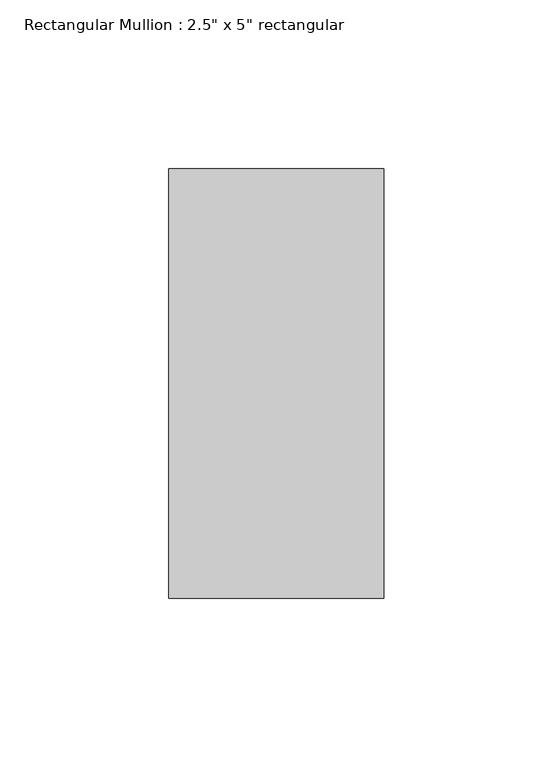
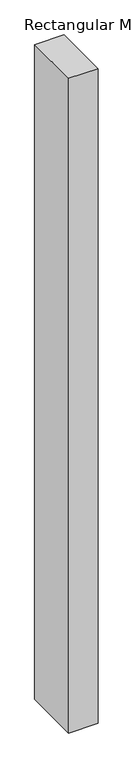
"""IFC4 building model written with IfcOpenShell, lengths in millimetres: member geometry."""

from ifc_helpers import new_model, si_unit, frame, origin, place, context, project, spatial, polyline, outline, extrude, source, transform, mapped, element, save


def member_241584b0(model_context):
    return source(origin(), model_context, "Body", "SweptSolid", [
        extrude(outline(polyline([(0.0, 63.5), (0.0, -63.5), (-63.5, -63.5), (-63.5, 63.5), (0.0, 63.5)])), frame((0.0, 0.0, -1493.5433028), z_axis=(0.0, 0.0, 1.0), x_axis=(1.0, 0.0, 0.0)), (0.0, 0.0, 1.0), 1493.5433028),
    ])


if __name__ == "__main__":
    model = new_model("IFC4")
    model_context = context("Model", 3, world=origin())
    ifc_project = project(units=[si_unit("LENGTHUNIT", "METRE", prefix="MILLI")], contexts=[model_context])
    site = spatial("IfcSite", under=ifc_project)
    building = spatial("IfcBuilding", under=site)
    placement = place(None, origin())
    member_shape = member_241584b0(model_context)
    element("IfcMember", 1, ObjectType="Rectangular Mullion : 2.5\" x 5\" rectangular", at=placement, inside=building, context=model_context, shape_type="MappedRepresentation", body=[
        mapped(member_shape, transform((0.0, 0.0, 0.0), x_axis=(1.0, 0.0, 0.0), y_axis=(0.0, 1.0, 0.0), z_axis=(0.0, 0.0, 1.0))),
    ])
    save(model, "model.ifc")

# Revit data of these elements
# Type "Rectangular Mullion : 2.5\" x 5\" rectangular"
#   built-in parameter 1007304 = 0.416667 (stored number, unit not read)
#   built-in parameter 1007301 = 0.104167 (stored number, unit not read)
#   built-in parameter 1007300 = 0.104167 (stored number, unit not read)
# Element 1 (IfcMember, "Rectangular Mullion : 2.5\" x 5\" rectangular")
#   Materials on its faces: "Aluminum"
# Materials
#   "Aluminum": class "Metal", colour RGB 247 247 247, transparency 0, Description = "Aluminum 6061", Cost = 0
